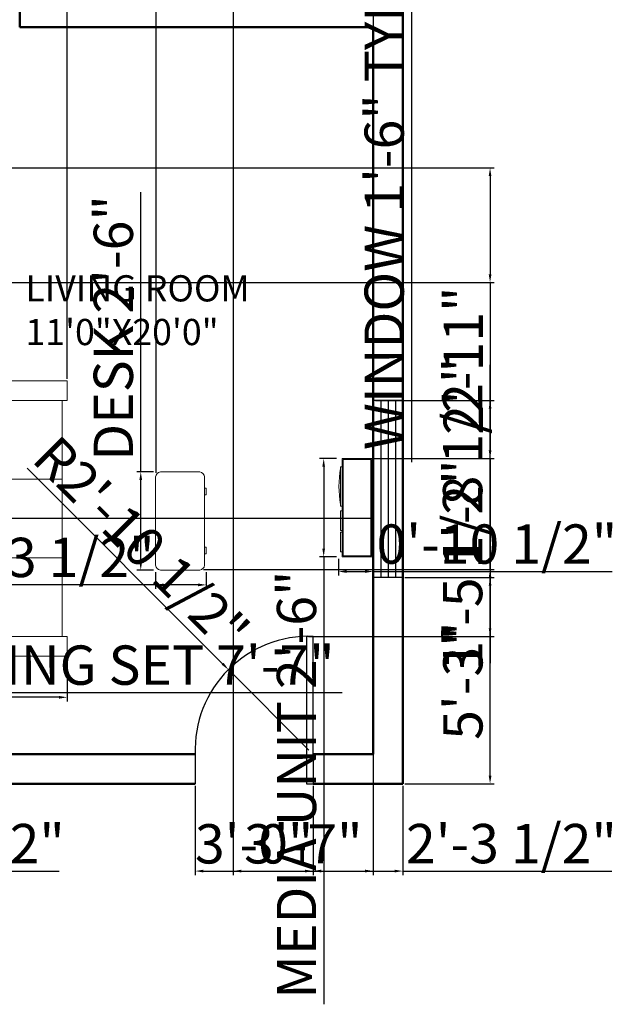
# Model space of a CAD drawing. Units: inches. Extents: x 2787 to 3354, y 1541 to 2259.
# Tile 2 of 3: x 3131 to 3312, y 1541 to 1842. Entities that reach past the tile are written whole.
import ezdxf

# ---------------------------------------------------------------- set-up
doc = ezdxf.new("R2010")
doc.units = ezdxf.units.IN
for name, color, linetype, lineweight in [('A-ANNO-DIMS', 2, 'Continuous', 18), ('A-AREA-IDEN', 7, 'Continuous', 25), ('A-DOOR', 4, 'Continuous', 25), ('A-FURN', 8, 'Continuous', 18), ('A-GLAZ', 4, 'Continuous', 25), ('A-WALL', 7, 'Continuous', 50)]:
    doc.layers.add(name, color=color, linetype=linetype, lineweight=lineweight)
doc.styles.get("Standard").update_dxf_attribs({"font": 'arial.ttf'})
doc.dimstyles.new('ISO-25', dxfattribs={"dimtxt": 12, "dimasz": 2.5, "dimexe": 1.25, "dimexo": 0.625, "dimtad": 1, "dimdec": 1, "dimlunit": 3, "dimtxsty": 'Standard', "dimcen": 2.5, "dimadec": 0, "dimazin": 0, "dimtfac": 1, "dimtdec": 1, "dimtmove": 0, "dimatfit": 3, "dimfxl": 1, "dimarcsym": 0})

# ---------------------------------------------------------------- blocks, each defined once
blk = doc.blocks.new('Window - Wood Frame 36 in. Wide plan')
for p, q in [((0, 6), (0, 0)), ((0, 4.5), (36, 4.5)), ((36, 6), (36, 0)), ((0, 3), (36, 3)), ((0, 1.5), (36, 1.5))]:
    blk.add_line(p, q)
blk = doc.blocks.new('Sofa - Roundback 7 ft.')
for p, q in [((-12.00002, -32.4421), (-12.00003, -6.5971)), ((11.99997, -32.4421), (11.99998, -6.5971)), ((-36.000027, -34), (-36.000027, -11.4696)), ((35.99998, -34), (35.99998, -11.4696)), ((-35.999844, -13.3819), (35.9998, -13.3819)), ((-36.000027, -32.4421), (35.99998, -32.4421))]:
    blk.add_line(p, q)
for points in [[(-36.000027, -34), (-42.000027, -34), (-42.000027, -8)], [(41.99998, -8), (41.99998, -34), (35.99998, -34)]]:
    blk.add_lwpolyline(points)
for centre, radius, start, end in [((0, -114.25), 114.25, 68.43141, 111.5686), ((-0.00001, -127.1968), 121.1968, 72.72033, 107.2797)]:
    blk.add_arc(centre, radius, start, end)
blk = doc.blocks.new('Entertainment Center')
for p, q in [((-4, 0), (-5, -1)), ((4, 0), (-4, 0)), ((5, -1), (4, 0)), ((-17, -19), (-17, -1)), ((-17, -1), (43, -1)), ((-16.5, -18.5), (-16.5, -1.5)), ((-16.5, -1.5), (42.5, -1.5)), ((42.5, -1.5), (42.5, -18.5)), ((43, -1), (43, -19)), ((43, -19), (-17, -19)), ((42.5, -18.5), (-16.5, -18.5)), ((-12, -20), (-12, -19)), ((12, -20), (-12, -20)), ((12, -19), (12, -20)), ((15, -20), (15, -19)), ((27, -20), (15, -20)), ((27, -19), (27, -20)), ((28, -20), (28, -19)), ((40, -20), (28, -20)), ((40, -19), (40, -20))]:
    blk.add_line(p, q)
blk.add_arc((0, 40), 61, 259.6111, 280.3889)
blk = doc.blocks.new('Desk - 30 x 60 in.')
for p, q in [((-26.999995, 0), (26.999995, 0)), ((-29.999995, -27), (-29.999995, -3)), ((29.999995, -3), (29.999995, -27)), ((26.999995, -30), (-26.999995, -30)), ((-20.000005, -30), (-20.000005, -31)), ((-16.000005, -31), (-16.000005, -30)), ((15.999995, -31), (15.999995, -30)), ((19.999995, -30), (19.999995, -31)), ((-20.000005, -31), (-16.000005, -31)), ((19.999995, -31), (15.999995, -31))]:
    blk.add_line(p, q)
for centre, start, end in [((-26.499995, -3.5), 98.1301, 171.8699), ((26.499995, -3.5), 8.130102, 81.8699), ((-26.499995, -26.5), 188.1301, 261.8699), ((26.499995, -26.5), 278.1301, 351.8699)]:
    blk.add_arc(centre, 3.535534, start, end)
blk = doc.blocks.new('*D14')
at = {"layer": 'A-ANNO-DIMS', "color": 0, "lineweight": -2, "transparency": 16777216}
for p, q in [((3248.65, 1880.03), (3251.97, 1880.03)), ((3250.72, 1877.53), (3250.72, 1864.53)), ((3248.65, 1862.03), (3251.97, 1862.03)), ((3250.72, 1862.03), (3250.72, 1706.43))]:
    blk.add_line(p, q, dxfattribs=at)
at = {"layer": 'A-ANNO-DIMS', "color": 0, "transparency": 16777216}
for points in [[(3250.31, 1877.53), (3251.14, 1877.53), (3250.72, 1880.03)], [(3250.31, 1864.53), (3251.14, 1864.53), (3250.72, 1862.03)]]:
    blk.add_solid(points, dxfattribs=at)
at = {"layer": 'Defpoints', "color": 0, "transparency": 16777216}
for p in [(3248.02, 1880.03), (3248.02, 1862.03), (3250.72, 1862.03)]:
    blk.add_point(p, dxfattribs=at)
at = {"layer": 'A-ANNO-DIMS', "color": 0, "transparency": 16777216, "insert": (3243.89, 1782.98), "char_height": 12, "attachment_point": 5, "rotation": 90}
blk.add_mtext('WINDOW 1\'-6" TYP.', dxfattribs=at)
blk = doc.blocks.new('*D24')
at = {"layer": 'A-ANNO-DIMS', "color": 0, "lineweight": -2, "transparency": 16777216}
for p, q in [((3002.87, 1649.12), (3002.87, 1634.84)), ((3093.87, 1649.12), (3093.87, 1634.84)), ((3005.37, 1636.09), (3091.37, 1636.09)), ((3093.87, 1636.09), (3229.51, 1636.09))]:
    blk.add_line(p, q, dxfattribs=at)
at = {"layer": 'A-ANNO-DIMS', "color": 0, "transparency": 16777216}
for points in [[(3005.37, 1636.51), (3005.37, 1635.68), (3002.87, 1636.09)], [(3091.37, 1636.51), (3091.37, 1635.68), (3093.87, 1636.09)]]:
    blk.add_solid(points, dxfattribs=at)
at = {"layer": 'Defpoints', "color": 0, "transparency": 16777216}
for p in [(3002.87, 1649.74), (3093.87, 1649.74), (3093.87, 1636.09)]:
    blk.add_point(p, dxfattribs=at)
at = {"layer": 'A-ANNO-DIMS', "color": 0, "transparency": 16777216, "insert": (3162.94, 1642.92), "char_height": 12, "attachment_point": 5}
blk.add_mtext('DINING SET 7\'-7"', dxfattribs=at)
blk = doc.blocks.new('*D27')
at = {"layer": 'A-ANNO-DIMS', "color": 0, "lineweight": -2, "transparency": 16777216}
for p, q in [((3108.86, 1646.64), (3108.86, 1633.41)), ((3145.52, 1646.64), (3145.52, 1633.41)), ((3108.86, 1634.66), (3045.25, 1634.66)), ((3143.02, 1634.66), (3111.36, 1634.66))]:
    blk.add_line(p, q, dxfattribs=at)
at = {"layer": 'A-ANNO-DIMS', "color": 0, "transparency": 16777216}
for points in [[(3111.36, 1635.08), (3111.36, 1634.24), (3108.86, 1634.66)], [(3143.02, 1635.08), (3143.02, 1634.24), (3145.52, 1634.66)]]:
    blk.add_solid(points, dxfattribs=at)
at = {"layer": 'Defpoints', "color": 0, "transparency": 16777216}
for p in [(3108.86, 1647.26), (3145.52, 1647.26), (3108.86, 1634.66)]:
    blk.add_point(p, dxfattribs=at)
at = {"layer": 'A-ANNO-DIMS', "color": 0, "transparency": 16777216, "insert": (3075.81, 1641.49), "char_height": 12, "attachment_point": 5}
blk.add_mtext('3\'-0 1/2"', dxfattribs=at)
blk = doc.blocks.new('*D28')
at = {"layer": 'A-ANNO-DIMS', "color": 0, "lineweight": -2, "transparency": 16777216}
for p, q in [((3227.73, 1707.55), (3222.61, 1707.55)), ((3223.86, 1705.05), (3223.86, 1680.05)), ((3227.73, 1677.55), (3222.61, 1677.55)), ((3223.86, 1677.55), (3223.86, 1540.94))]:
    blk.add_line(p, q, dxfattribs=at)
at = {"layer": 'A-ANNO-DIMS', "color": 0, "transparency": 16777216}
for points in [[(3223.44, 1705.05), (3224.27, 1705.05), (3223.86, 1707.55)], [(3223.44, 1680.05), (3224.27, 1680.05), (3223.86, 1677.55)]]:
    blk.add_solid(points, dxfattribs=at)
at = {"layer": 'Defpoints', "color": 0, "transparency": 16777216}
for p in [(3228.36, 1707.55), (3223.86, 1677.55), (3228.36, 1677.55)]:
    blk.add_point(p, dxfattribs=at)
at = {"layer": 'A-ANNO-DIMS', "color": 0, "transparency": 16777216, "insert": (3217.11, 1608), "char_height": 12, "attachment_point": 5, "rotation": 90}
blk.add_mtext('MEDIA UNIT 2\'-6"', dxfattribs=at)
blk = doc.blocks.new('*D29')
at = {"layer": 'A-ANNO-DIMS', "color": 0, "lineweight": -2, "transparency": 16777216}
for p, q in [((3228.36, 1676.93), (3228.36, 1671.8)), ((3239.02, 1676.93), (3239.02, 1671.8)), ((3230.86, 1673.05), (3236.52, 1673.05)), ((3239.02, 1673.05), (3311.96, 1673.05))]:
    blk.add_line(p, q, dxfattribs=at)
at = {"layer": 'A-ANNO-DIMS', "color": 0, "transparency": 16777216}
for points in [[(3230.86, 1673.47), (3230.86, 1672.64), (3228.36, 1673.05)], [(3236.52, 1673.47), (3236.52, 1672.64), (3239.02, 1673.05)]]:
    blk.add_solid(points, dxfattribs=at)
at = {"layer": 'Defpoints', "color": 0, "transparency": 16777216}
for p in [(3228.36, 1677.55), (3239.02, 1677.55), (3239.02, 1673.05)]:
    blk.add_point(p, dxfattribs=at)
at = {"layer": 'A-ANNO-DIMS', "color": 0, "transparency": 16777216, "insert": (3276.74, 1679.88), "char_height": 12, "attachment_point": 5}
blk.add_mtext('0\'-10 1/2"', dxfattribs=at)
blk = doc.blocks.new('*D30')
at = {"layer": 'A-ANNO-DIMS', "color": 0, "lineweight": -2, "transparency": 16777216}
for p, q in [((3168, 1703.47), (3168, 1788.83)), ((3171.87, 1703.47), (3166.75, 1703.47)), ((3168, 1675.97), (3168, 1700.97)), ((3171.87, 1673.47), (3166.75, 1673.47))]:
    blk.add_line(p, q, dxfattribs=at)
at = {"layer": 'A-ANNO-DIMS', "color": 0, "transparency": 16777216}
for points in [[(3167.58, 1700.97), (3168.42, 1700.97), (3168, 1703.47)], [(3167.58, 1675.97), (3168.42, 1675.97), (3168, 1673.47)]]:
    blk.add_solid(points, dxfattribs=at)
at = {"layer": 'Defpoints', "color": 0, "transparency": 16777216}
for p in [(3168, 1703.47), (3172.5, 1703.47), (3172.5, 1673.47)]:
    blk.add_point(p, dxfattribs=at)
at = {"layer": 'A-ANNO-DIMS', "color": 0, "transparency": 16777216, "insert": (3161.17, 1747.4), "char_height": 12, "attachment_point": 5, "rotation": 90}
blk.add_mtext('DESK 2\'-6"', dxfattribs=at)
blk = doc.blocks.new('*D31')
at = {"layer": 'A-ANNO-DIMS', "color": 0, "lineweight": -2, "transparency": 16777216}
for p, q in [((3172.5, 1672.84), (3172.5, 1667.72)), ((3188, 1672.84), (3188, 1667.72)), ((3172.5, 1668.97), (3110.02, 1668.97)), ((3185.5, 1668.97), (3175, 1668.97))]:
    blk.add_line(p, q, dxfattribs=at)
at = {"layer": 'A-ANNO-DIMS', "color": 0, "transparency": 16777216}
for points in [[(3175, 1669.39), (3175, 1668.55), (3172.5, 1668.97)], [(3185.5, 1669.39), (3185.5, 1668.55), (3188, 1668.97)]]:
    blk.add_solid(points, dxfattribs=at)
at = {"layer": 'Defpoints', "color": 0, "transparency": 16777216}
for p in [(3172.5, 1673.47), (3188, 1673.47), (3172.5, 1668.97)]:
    blk.add_point(p, dxfattribs=at)
at = {"layer": 'A-ANNO-DIMS', "color": 0, "transparency": 16777216, "insert": (3140.01, 1675.8), "char_height": 12, "attachment_point": 5}
blk.add_mtext('1\'-3 1/2"', dxfattribs=at)
blk = doc.blocks.new('*D39')
at = {"layer": 'A-ANNO-DIMS', "color": 0, "lineweight": -2, "transparency": 16777216}
for p, q in [((3248.65, 1671.24), (3275.92, 1671.24)), ((3274.67, 1610.76), (3274.67, 1668.74)), ((3248.65, 1608.26), (3275.92, 1608.26))]:
    blk.add_line(p, q, dxfattribs=at)
at = {"layer": 'A-ANNO-DIMS', "color": 0, "transparency": 16777216}
for points in [[(3274.26, 1668.74), (3275.09, 1668.74), (3274.67, 1671.24)], [(3274.26, 1610.76), (3275.09, 1610.76), (3274.67, 1608.26)]]:
    blk.add_solid(points, dxfattribs=at)
at = {"layer": 'Defpoints', "color": 0, "transparency": 16777216}
for p in [(3248.02, 1671.24), (3274.67, 1671.24), (3248.02, 1608.26)]:
    blk.add_point(p, dxfattribs=at)
at = {"layer": 'A-ANNO-DIMS', "color": 0, "transparency": 16777216, "insert": (3267.92, 1639.75), "char_height": 12, "attachment_point": 5, "rotation": 90}
blk.add_mtext('5\'-3"', dxfattribs=at)
blk = doc.blocks.new('*D41')
at = {"layer": 'A-ANNO-DIMS', "color": 0, "lineweight": -2, "transparency": 16777216}
for p, q in [((3184.62, 1607.64), (3184.62, 1580.36)), ((3220.62, 1607.64), (3220.62, 1580.36)), ((3187.12, 1581.61), (3218.12, 1581.61))]:
    blk.add_line(p, q, dxfattribs=at)
at = {"layer": 'A-ANNO-DIMS', "color": 0, "transparency": 16777216}
for points in [[(3187.12, 1582.03), (3187.12, 1581.19), (3184.62, 1581.61)], [(3218.12, 1582.03), (3218.12, 1581.19), (3220.62, 1581.61)]]:
    blk.add_solid(points, dxfattribs=at)
at = {"layer": 'Defpoints', "color": 0, "transparency": 16777216}
for p in [(3184.62, 1608.26), (3220.62, 1608.26), (3220.62, 1581.61)]:
    blk.add_point(p, dxfattribs=at)
at = {"layer": 'A-ANNO-DIMS', "color": 0, "transparency": 16777216, "insert": (3202.62, 1588.37), "char_height": 12, "attachment_point": 5}
blk.add_mtext('3\'-0"', dxfattribs=at)
blk = doc.blocks.new('*D42')
at = {"layer": 'A-ANNO-DIMS', "color": 0, "lineweight": -2, "transparency": 16777216}
for p, q in [((3220.62, 1607.64), (3220.62, 1580.36)), ((3248.02, 1607.64), (3248.02, 1580.36)), ((3223.12, 1581.61), (3245.52, 1581.61)), ((3248.02, 1581.61), (3311.84, 1581.61))]:
    blk.add_line(p, q, dxfattribs=at)
at = {"layer": 'A-ANNO-DIMS', "color": 0, "transparency": 16777216}
for points in [[(3223.12, 1582.03), (3223.12, 1581.19), (3220.62, 1581.61)], [(3245.52, 1582.03), (3245.52, 1581.19), (3248.02, 1581.61)]]:
    blk.add_solid(points, dxfattribs=at)
at = {"layer": 'Defpoints', "color": 0, "transparency": 16777216}
for p in [(3220.62, 1608.26), (3248.02, 1608.26), (3248.02, 1581.61)]:
    blk.add_point(p, dxfattribs=at)
at = {"layer": 'A-ANNO-DIMS', "color": 0, "transparency": 16777216, "insert": (3281.18, 1588.44), "char_height": 12, "attachment_point": 5}
blk.add_mtext('2\'-3 1/2"', dxfattribs=at)
blk = doc.blocks.new('*D47')
at = {"layer": 'A-ANNO-DIMS', "color": 0, "lineweight": -2, "transparency": 16777216}
for p, q in [((3072.52, 2078.64), (3072.52, 1580.36)), ((3077.02, 2078.64), (3077.02, 1580.36)), ((3070.02, 1581.61), (3067.52, 1581.61)), ((3072.52, 1581.61), (3077.02, 1581.61)), ((3079.52, 1581.61), (3143.13, 1581.61))]:
    blk.add_line(p, q, dxfattribs=at)
at = {"layer": 'A-ANNO-DIMS', "color": 0, "transparency": 16777216}
for points in [[(3070.02, 1582.03), (3070.02, 1581.19), (3072.52, 1581.61)], [(3079.52, 1582.03), (3079.52, 1581.19), (3077.02, 1581.61)]]:
    blk.add_solid(points, dxfattribs=at)
at = {"layer": 'Defpoints', "color": 0, "transparency": 16777216}
for p in [(3072.52, 2079.26), (3077.02, 2079.26), (3077.02, 1581.61)]:
    blk.add_point(p, dxfattribs=at)
at = {"layer": 'A-ANNO-DIMS', "color": 0, "transparency": 16777216, "insert": (3112.58, 1588.44), "char_height": 12, "attachment_point": 5}
blk.add_mtext('0\'-4 1/2"', dxfattribs=at)
blk = doc.blocks.new('*D48')
at = {"layer": 'A-ANNO-DIMS', "color": 0, "lineweight": -2, "transparency": 16777216}
for p, q in [((3032.73, 1796.26), (3275.92, 1796.26)), ((3274.67, 1793.76), (3274.67, 1763.76)), ((3032.73, 1761.26), (3275.92, 1761.26)), ((3274.67, 1761.26), (3274.67, 1716.08))]:
    blk.add_line(p, q, dxfattribs=at)
at = {"layer": 'A-ANNO-DIMS', "color": 0, "transparency": 16777216}
for points in [[(3274.26, 1793.76), (3275.09, 1793.76), (3274.67, 1796.26)], [(3274.26, 1763.76), (3275.09, 1763.76), (3274.67, 1761.26)]]:
    blk.add_solid(points, dxfattribs=at)
at = {"layer": 'Defpoints', "color": 0, "transparency": 16777216}
for p in [(3032.1, 1796.26), (3032.1, 1761.26), (3274.67, 1761.26)]:
    blk.add_point(p, dxfattribs=at)
at = {"layer": 'A-ANNO-DIMS', "color": 0, "transparency": 16777216, "insert": (3268.02, 1737.42), "char_height": 12, "attachment_point": 5, "rotation": 90}
blk.add_mtext('2\'-11"', dxfattribs=at)
blk = doc.blocks.new('*D51')
at = {"layer": 'A-ANNO-DIMS', "color": 0, "lineweight": -2, "transparency": 16777216}
for p, q in [((3196.24, 2078.43), (3196.24, 1580.36)), ((3239.02, 2078.64), (3239.02, 1580.36)), ((3198.74, 1581.61), (3236.52, 1581.61))]:
    blk.add_line(p, q, dxfattribs=at)
at = {"layer": 'A-ANNO-DIMS', "color": 0, "transparency": 16777216}
for points in [[(3198.74, 1582.03), (3198.74, 1581.19), (3196.24, 1581.61)], [(3236.52, 1582.03), (3236.52, 1581.19), (3239.02, 1581.61)]]:
    blk.add_solid(points, dxfattribs=at)
at = {"layer": 'Defpoints', "color": 0, "transparency": 16777216}
for p in [(3196.24, 2079.05), (3239.02, 2079.26), (3239.02, 1581.61)]:
    blk.add_point(p, dxfattribs=at)
at = {"layer": 'A-ANNO-DIMS', "color": 0, "transparency": 16777216, "insert": (3217.63, 1588.37), "char_height": 12, "attachment_point": 5}
blk.add_mtext('3\'-7"', dxfattribs=at)
blk = doc.blocks.new('*D56')
at = {"layer": 'A-ANNO-DIMS', "color": 0, "lineweight": -2, "transparency": 16777216}
for p, q in [((3145.52, 1731.89), (3145.52, 2116.16)), ((3172.67, 1703.14), (3172.67, 2116.16)), ((3148.02, 2114.91), (3170.17, 2114.91)), ((3172.67, 2114.91), (3208.53, 2114.91))]:
    blk.add_line(p, q, dxfattribs=at)
at = {"layer": 'A-ANNO-DIMS', "color": 0, "transparency": 16777216}
for points in [[(3148.02, 2115.33), (3148.02, 2114.49), (3145.52, 2114.91)], [(3170.17, 2115.33), (3170.17, 2114.49), (3172.67, 2114.91)]]:
    blk.add_solid(points, dxfattribs=at)
at = {"layer": 'Defpoints', "color": 0, "transparency": 16777216}
for p in [(3172.67, 2114.91), (3145.52, 1731.26), (3172.67, 1702.52)]:
    blk.add_point(p, dxfattribs=at)
at = {"layer": 'A-ANNO-DIMS', "color": 0, "transparency": 16777216, "insert": (3191.85, 2121.67), "char_height": 12, "attachment_point": 5}
blk.add_mtext('2\'-3"', dxfattribs=at)
blk = doc.blocks.new('*D57')
at = {"layer": 'A-ANNO-DIMS', "color": 0, "lineweight": -2, "transparency": 16777216}
for p, q in [((3239.65, 1725.24), (3275.92, 1725.24)), ((3274.67, 1722.74), (3274.67, 1710.05)), ((3239.15, 1707.55), (3275.92, 1707.55)), ((3274.67, 1707.55), (3274.67, 1645.07))]:
    blk.add_line(p, q, dxfattribs=at)
at = {"layer": 'A-ANNO-DIMS', "color": 0, "transparency": 16777216}
for points in [[(3274.26, 1722.74), (3275.09, 1722.74), (3274.67, 1725.24)], [(3274.26, 1710.05), (3275.09, 1710.05), (3274.67, 1707.55)]]:
    blk.add_solid(points, dxfattribs=at)
at = {"layer": 'Defpoints', "color": 0, "transparency": 16777216}
for p in [(3239.02, 1725.24), (3238.52, 1707.55), (3274.67, 1707.55)]:
    blk.add_point(p, dxfattribs=at)
at = {"layer": 'A-ANNO-DIMS', "color": 0, "transparency": 16777216, "insert": (3267.84, 1675.06), "char_height": 12, "attachment_point": 5, "rotation": 90}
blk.add_mtext('1\'-5 1/2"', dxfattribs=at)
blk = doc.blocks.new('*D58')
at = {"layer": 'A-ANNO-DIMS', "color": 0, "lineweight": -2, "transparency": 16777216}
for p, q in [((3274.67, 1673.64), (3274.67, 1736.12)), ((3187.17, 1673.64), (3275.92, 1673.64)), ((3274.67, 1655.76), (3274.67, 1671.14)), ((3219.25, 1653.26), (3275.92, 1653.26))]:
    blk.add_line(p, q, dxfattribs=at)
at = {"layer": 'A-ANNO-DIMS', "color": 0, "transparency": 16777216}
for points in [[(3274.26, 1671.14), (3275.09, 1671.14), (3274.67, 1673.64)], [(3274.26, 1655.76), (3275.09, 1655.76), (3274.67, 1653.26)]]:
    blk.add_solid(points, dxfattribs=at)
at = {"layer": 'Defpoints', "color": 0, "transparency": 16777216}
for p in [(3186.55, 1673.64), (3274.67, 1673.64), (3218.62, 1653.26)]:
    blk.add_point(p, dxfattribs=at)
at = {"layer": 'A-ANNO-DIMS', "color": 0, "transparency": 16777216, "insert": (3267.84, 1706.13), "char_height": 12, "attachment_point": 5, "rotation": 90}
blk.add_mtext('1\'-8 1/2"', dxfattribs=at)
blk = doc.blocks.new('*D59')
at = {"layer": 'A-ANNO-DIMS', "color": 0, "lineweight": -2, "transparency": 16777216}
for p, q in [((3133.31, 1704.58), (3193, 1644.88)), ((3219.32, 1618.56), (3194.77, 1643.11))]:
    blk.add_line(p, q, dxfattribs=at)
at = {"layer": 'A-ANNO-DIMS', "color": 0, "transparency": 16777216}
blk.add_solid([(3193.3, 1645.18), (3192.71, 1644.59), (3194.77, 1643.11)], dxfattribs=at)
at = {"layer": 'Defpoints', "color": 0, "transparency": 16777216}
for p in [(3194.77, 1643.11), (3219.32, 1618.56)]:
    blk.add_point(p, dxfattribs=at)
at = {"layer": 'A-ANNO-DIMS', "color": 0, "transparency": 16777216, "insert": (3167.1, 1680.44), "char_height": 12, "attachment_point": 5, "rotation": 314.9998}
blk.add_mtext('R2\'-10 1/2"', dxfattribs=at)
blk = doc.blocks.new('*D63')
at = {"layer": 'A-ANNO-DIMS', "color": 0, "lineweight": -2, "transparency": 16777216}
for p, q in [((3017.83, 1689.26), (3115.02, 1689.26)), ((3238.72, 1689.26), (3117.52, 1689.26))]:
    blk.add_line(p, q, dxfattribs=at)
at = {"layer": 'A-ANNO-DIMS', "color": 0, "transparency": 16777216}
blk.add_solid([(3115.02, 1689.68), (3115.02, 1688.84), (3117.52, 1689.26)], dxfattribs=at)
at = {"layer": 'Defpoints', "color": 0, "transparency": 16777216}
for p in [(3117.52, 1689.26), (3238.72, 1689.26)]:
    blk.add_point(p, dxfattribs=at)
at = {"layer": 'A-ANNO-DIMS', "color": 0, "transparency": 16777216, "insert": (3044.81, 1696.01), "char_height": 12, "attachment_point": 5}
blk.add_mtext('R10\'-1"', dxfattribs=at)
blk = doc.blocks.new('*D64')
at = {"layer": 'A-ANNO-DIMS', "color": 0, "lineweight": -2, "transparency": 16777216}
for p, q in [((3006.68, 1689.26), (3109.02, 1689.26)), ((3225.77, 1689.26), (3111.52, 1689.26))]:
    blk.add_line(p, q, dxfattribs=at)
at = {"layer": 'A-ANNO-DIMS', "color": 0, "transparency": 16777216}
blk.add_solid([(3109.02, 1689.68), (3109.02, 1688.84), (3111.52, 1689.26)], dxfattribs=at)
at = {"layer": 'Defpoints', "color": 0, "transparency": 16777216}
for p in [(3111.52, 1689.26), (3225.77, 1689.26)]:
    blk.add_point(p, dxfattribs=at)
at = {"layer": 'A-ANNO-DIMS', "color": 0, "transparency": 16777216, "insert": (3042.97, 1696.09), "char_height": 12, "attachment_point": 5}
blk.add_mtext('R9\'-6 1/2"', dxfattribs=at)

msp = doc.modelspace()

# ---------------------------------------------------------------- linework, layer by layer
at = {"layer": 'A-DOOR'}
for p, q in [((3220.62, 1653.26), (3218.62, 1653.26)), ((3218.62, 1653.26), (3218.62, 1608.26)), ((3220.62, 1617.26), (3220.62, 1653.26)), ((3184.62, 1617.26), (3184.62, 1608.26)), ((3220.62, 1617.26), (3220.62, 1608.26)), ((3218.62, 1608.26), (3220.62, 1608.26))]:
    msp.add_line(p, q, dxfattribs=at)
msp.add_arc((3219.32, 1618.56), 34.73, 87.8558, 182.1442, dxfattribs=at)
at = {"layer": 'A-WALL'}
for p, q in [((3248.02, 2088.26), (3248.02, 1608.26)), ((3131.02, 1911.26), (3131.02, 1839.26)), ((3131.02, 1839.26), (3239.02, 1839.26)), ((3239.02, 1839.26), (3239.02, 1617.26)), ((3184.62, 1617.26), (2993.02, 1617.26)), ((3239.02, 1617.26), (3220.62, 1617.26)), ((3184.62, 1608.26), (2888.02, 1608.26)), ((3248.02, 1608.26), (3220.62, 1608.26))]:
    msp.add_line(p, q, dxfattribs=at)

# ---------------------------------------------------------------- block references
at = {"layer": 'A-FURN', "rotation": 90}
msp.add_blockref('Sofa - Roundback 7 ft.', (3111.52, 1689.26), dxfattribs=at)
at = {"layer": 'A-FURN', "xscale": 0.5, "yscale": 0.5, "zscale": 0.5}
for name, p, rotation in [('Entertainment Center', (3239.02, 1699.05), 270), ('Desk - 30 x 60 in.', (3172.5, 1688.47), 90)]:
    msp.add_blockref(name, p, dxfattribs=dict(at, rotation=rotation))
at = {"layer": 'A-GLAZ', "xscale": 1.5, "yscale": 1.5, "zscale": 1.5, "rotation": 270}
msp.add_blockref('Window - Wood Frame 36 in. Wide plan', (3239.02, 1725.24), dxfattribs=at)

# ---------------------------------------------------------------- texts
at = {"layer": 'A-AREA-IDEN', "insert": (3132.77, 1763.5), "char_height": 8, "attachment_point": 1}
msp.add_mtext_dynamic_manual_height_columns('LIVING ROOM\\P11\'0"X20\'0"', width=129.1776, gutter_width=12.5, heights=[0], dxfattribs=at)

# ---------------------------------------------------------------- dimensions: what is measured, and where the dimension line sits
at = {"layer": 'A-ANNO-DIMS'}
for base, p1, p2, picture, middle in [((3172.6713, 2114.911), (3145.524, 1731.2609), (3172.6713, 1702.5155), '*D56', (3191.8482, 2121.6669)), ((3077.02, 1581.61), (3072.52, 2079.26), (3077.02, 2079.26), '*D47', (3112.58, 1588.44)), ((3239.02, 1581.61), (3196.24, 2079.05), (3239.02, 2079.26), '*D51', (3217.63, 1588.37)), ((3239.02, 1673.05), (3228.36, 1677.55), (3239.02, 1677.55), '*D29', (3276.74, 1679.88)), ((3220.62, 1581.61), (3184.62, 1608.26), (3220.62, 1608.26), '*D41', (3202.62, 1588.37)), ((3248.02, 1581.61), (3220.62, 1608.26), (3248.02, 1608.26), '*D42', (3281.18, 1588.44))]:
    dim = msp.add_linear_dim(base=base, p1=p1, p2=p2, dimstyle='ISO-25', override={"dimdec": 1, "dimlfac": 1, "dimrnd": 0, "dimzin": 1, "dimdsep": 46, "dimlunit": 4, "dimfrac": 2}, dxfattribs=at)
    dim.commit()
    dim.dimension.update_dxf_attribs({"geometry": picture, "text_midpoint": middle})
for base, p1, p2, angle, text, picture, middle in [((3250.72, 1862.03), (3248.02, 1880.03), (3248.02, 1862.03), 270, 'WINDOW <> TYP.', '*D14', (3243.89, 1782.98)), ((3168, 1703.47), (3172.5, 1673.47), (3172.5, 1703.47), 90, 'DESK <>', '*D30', (3161.17, 1747.4)), ((3223.86, 1677.55), (3228.36, 1707.55), (3228.36, 1677.55), 270, 'MEDIA UNIT <>', '*D28', (3217.11, 1608))]:
    dim = msp.add_linear_dim(base=base, p1=p1, p2=p2, angle=angle, text=text, dimstyle='ISO-25', override={"dimdec": 1, "dimlfac": 1, "dimrnd": 0, "dimzin": 1, "dimdsep": 46, "dimlunit": 4, "dimfrac": 2}, dxfattribs=at)
    dim.commit()
    dim.dimension.update_dxf_attribs({"geometry": picture, "text_midpoint": middle})
for base, p1, p2, angle, picture, middle in [((3274.67, 1761.26), (3032.1, 1796.26), (3032.1, 1761.26), 90, '*D48', (3268.02, 1737.42)), ((3274.67, 1673.64), (3218.62, 1653.26), (3186.55, 1673.64), 90, '*D58', (3267.84, 1706.13)), ((3274.67, 1707.55), (3239.02, 1725.24), (3238.52, 1707.55), 90, '*D57', (3267.84, 1675.06)), ((3172.5, 1668.97), (3188, 1673.47), (3172.5, 1673.47), 180, '*D31', (3140.01, 1675.8)), ((3274.67, 1671.24), (3248.02, 1608.26), (3248.02, 1671.24), 90, '*D39', (3267.92, 1639.75)), ((3108.86, 1634.66), (3145.52, 1647.26), (3108.86, 1647.26), 180, '*D27', (3075.81, 1641.49))]:
    dim = msp.add_linear_dim(base=base, p1=p1, p2=p2, angle=angle, dimstyle='ISO-25', override={"dimdec": 1, "dimlfac": 1, "dimrnd": 0, "dimzin": 1, "dimdsep": 46, "dimlunit": 4, "dimfrac": 2}, dxfattribs=at)
    dim.commit()
    dim.dimension.update_dxf_attribs({"geometry": picture, "text_midpoint": middle})
for center, mpoint, picture, middle in [((3225.77398, 1689.260969), (3111.52398, 1689.261), '*D64', (3042.97398, 1689.261)), ((3238.72, 1689.26), (3117.52, 1689.26), '*D63', (3044.81, 1689.26))]:
    dim = msp.add_radius_dim(center=center, mpoint=mpoint, dimstyle='ISO-25', override={"dimdec": 1, "dimlfac": 1, "dimrnd": 0, "dimzin": 1, "dimdsep": 46, "dimlunit": 4, "dimfrac": 2}, dxfattribs=at)
    dim.commit()
    dim.dimension.update_dxf_attribs({"geometry": picture, "text_midpoint": middle, "dimtype": 164})
dim = msp.add_radius_dim(center=(3219.32, 1618.56), mpoint=(3194.77, 1643.11), dimstyle='ISO-25', override={"dimdec": 1, "dimlfac": 1, "dimrnd": 0, "dimzin": 1, "dimdsep": 46, "dimlunit": 4, "dimfrac": 2}, dxfattribs=at)
dim.commit()
dim.dimension.update_dxf_attribs({"geometry": '*D59', "text_midpoint": (3167.1, 1680.44)})
dim = msp.add_linear_dim(base=(3093.87, 1636.09), p1=(3002.87, 1649.74), p2=(3093.87, 1649.74), text='DINING SET <>', dimstyle='ISO-25', override={"dimdec": 1, "dimlfac": 1, "dimrnd": 0, "dimzin": 1, "dimdsep": 46, "dimlunit": 4, "dimfrac": 2}, dxfattribs=at)
dim.commit()
dim.dimension.update_dxf_attribs({"geometry": '*D24', "text_midpoint": (3162.94, 1642.92)})

doc.saveas('drawing.dxf')
